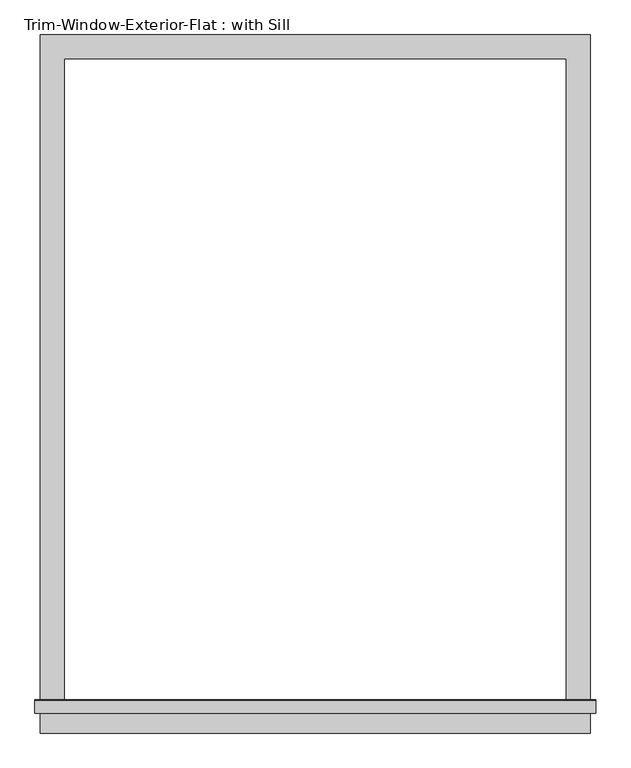
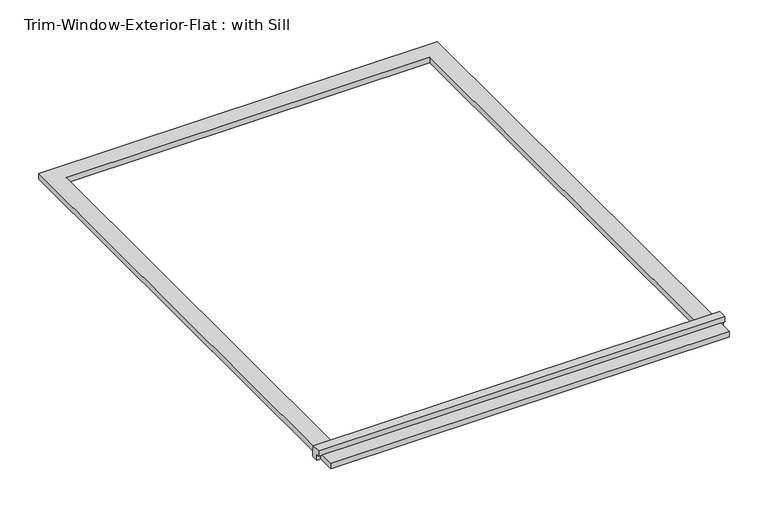
"""IFC4 building model written with IfcOpenShell, lengths in millimetres: proxy geometry, Trim-Window-Exterior-Flat : with Sill."""

from ifc_helpers import new_model, si_unit, frame, origin, origin_with_axes, place, context, project, spatial, polyline, outline, extrude, source, transform, mapped, element, save


def trim_window_exterior_flat_with_sill_c3105ee7(model_context):
    return source(origin(), model_context, "Body", "SweptSolid", [
        extrude(outline(polyline([(654.05, -1546.1823709), (654.05, -1603.3323709), (-654.05, -1603.3323709), (-654.05, -1546.1823709), (654.05, -1546.1823709)])), origin_with_axes(), (0.0, 0.0, 1.0), 19.05),
        extrude(outline(polyline([(-1555.75, 38.1), (-1526.4580645, 38.1), (-1524.0, 19.05), (-1524.0, 0.0), (-1546.1823709, 0.0), (-1546.1823709, 19.05), (-1555.75, 19.05), (-1555.75, 38.1)])), frame((-666.75, 0.0, 0.0), z_axis=(1.0, 0.0, 0.0), x_axis=(0.0, 1.0, 0.0)), (0.0, 0.0, 1.0), 1333.5),
        extrude(outline(polyline([(-654.05, 57.15), (654.05, 57.15), (654.05, -1524.0), (596.9, -1524.0), (596.9, 0.0), (-596.9, 0.0), (-596.9, -1524.0), (-654.05, -1524.0), (-654.05, 57.15)])), origin_with_axes(), (0.0, 0.0, 1.0), 19.05),
    ])


if __name__ == "__main__":
    model = new_model("IFC4")
    model_context = context("Model", 3, world=origin())
    ifc_project = project(units=[si_unit("LENGTHUNIT", "METRE", prefix="MILLI")], contexts=[model_context])
    site = spatial("IfcSite", under=ifc_project)
    building = spatial("IfcBuilding", under=site)
    placement = place(None, origin())
    trim_window_exterior_flat_with_sill_shape = trim_window_exterior_flat_with_sill_c3105ee7(model_context)
    element("IfcBuildingElementProxy", 1, Name="Trim-Window-Exterior-Flat : with Sill", ObjectType="Trim-Window-Exterior-Flat : with Sill", at=placement, inside=building, context=model_context, shape_type="MappedRepresentation", body=[
        mapped(trim_window_exterior_flat_with_sill_shape, transform((0.0, 0.0, 0.0), x_axis=(1.0, 0.0, 0.0), y_axis=(0.0, 1.0, 0.0), z_axis=(0.0, 0.0, 1.0))),
    ])
    save(model, "model.ifc")

# Revit data of these elements
# Type "Trim-Window-Exterior-Flat : with Sill"
#   Trim Width = 0' - 2 1/4"
#   Trim Thickness_Picture Frame = 0' - 1 1/4"
#   Trim Thickness_with Sill = 0' - 0 3/4"
#   Sill Thickness = 0' - 1 1/4"
#   Opening Width [instance default] = 2' - 0"
#   Opening Height [instance default] = 3' - 0"
#   Default Elevation = 4' - 0"
#   Sill = yes
#   Picture Frame = no
#   Trim Material [instance default] = none
# Element 1 (IfcBuildingElementProxy, "Trim-Window-Exterior-Flat : with Sill")
#   Opening Width = 3' - 11"
#   Opening Height = 5' - 0"
#   Trim Material = Clad - White
#   Materials on its faces: "Clad - White"
# Materials
#   "Clad - White": class "Wood", colour RGB 242 242 238, transparency 0, Cost = 0
